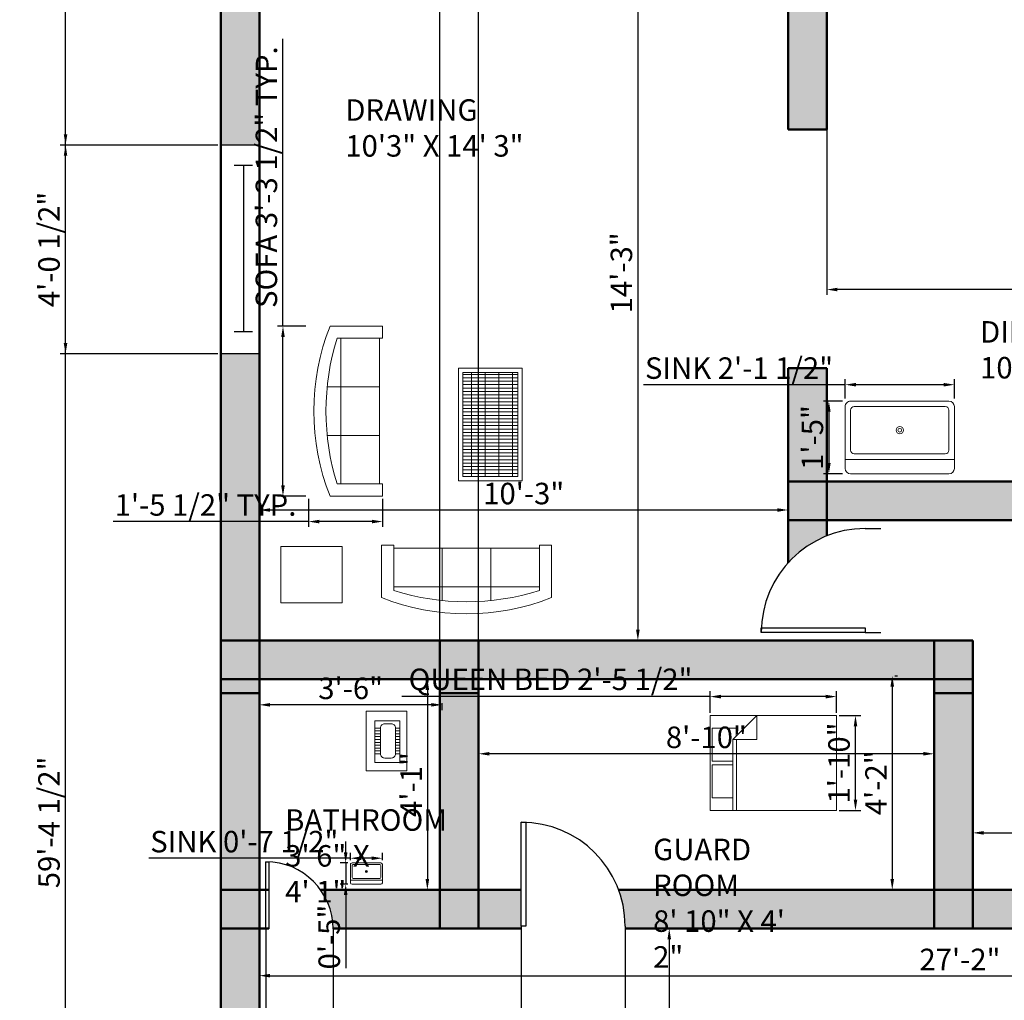
# Model space of a CAD drawing. Units: millimetres. Extents: x 2784 to 3697, y 603 to 1406.
# Tile 2 of 10: x 2784 to 3013, y 959 to 1187. Entities that reach past the tile are written whole.
import ezdxf

# ---------------------------------------------------------------- set-up
doc = ezdxf.new("R2010")
doc.units = ezdxf.units.MM
for name, color, linetype, lineweight in [('A-ANNO-DIMS', 140, 'Continuous', 18), ('A-AREA-IDEN', 150, 'Continuous', 25), ('A-DOOR', 10, 'Continuous', 25), ('A-FLOR-FIXT', 8, 'Continuous', 18), ('A-FURN', 80, 'Continuous', 18), ('A-GLAZ', 30, 'Continuous', 25), ('A-WALL', 2, 'Continuous', 50), ('A-WALL-PATT', 8, 'Continuous', 13)]:
    doc.layers.add(name, color=color, linetype=linetype, lineweight=lineweight)
doc.styles.get("Standard").update_dxf_attribs({"font": 'arial.ttf'})
doc.dimstyles.new('ISO-25', dxfattribs={"dimtxt": 5, "dimasz": 2.5, "dimexe": 1.25, "dimexo": 0.625, "dimtad": 1, "dimdec": 0, "dimlunit": 3, "dimtxsty": 'Standard', "dimcen": 2.5, "dimadec": 0, "dimazin": 0, "dimtfac": 1, "dimtdec": 0, "dimtmove": 0, "dimatfit": 3, "dimfxl": 1, "dimarcsym": 0})

# ---------------------------------------------------------------- blocks, each defined once
blk = doc.blocks.new('*U2')
for p, q in [((0, 0), (0, -6)), ((40, 0), (40, -6))]:
    blk.add_line(p, q)
blk.add_lwpolyline([(0, 0), (0, 40), (1.75, 40), (1.75, 0)], close=True)
blk.add_arc((0, 0), 40, 0, 90)
blk = doc.blocks.new('*U4')
for p, q in [((0, 4), (0, 0)), ((36, 4), (36, 0)), ((0, 2), (36, 2))]:
    blk.add_line(p, q)
blk = doc.blocks.new('Sofa - Roundback 7 ft.')
for p, q in [((-12.00002, -32.4421), (-12.00003, -6.5971)), ((11.99997, -32.4421), (11.99998, -6.5971)), ((-36.000027, -34), (-36.000027, -11.4696)), ((-35.999844, -13.3819), (35.9998, -13.3819)), ((35.99998, -34), (35.99998, -11.4696)), ((-36.000027, -32.4421), (35.99998, -32.4421))]:
    blk.add_line(p, q)
for points in [[(-36.000027, -34), (-42.000027, -34), (-42.000027, -8)], [(41.99998, -8), (41.99998, -34), (35.99998, -34)]]:
    blk.add_lwpolyline(points)
for centre, radius, start, end in [((0, -114.25), 114.25, 68.43141, 111.5686), ((-0.00001, -127.1968), 121.1968, 72.72033, 107.2797)]:
    blk.add_arc(centre, radius, start, end)
blk = doc.blocks.new('Sink-single - 30 in top')
blk.add_line((-15, -3.999996), (15, -3.999996))
for points in [[(-13.5, 0), (13.5, 0)], [(-15, -18.499996), (-15, -1.5)], [(15, -1.5), (15, -18.499996)], [(-13.5, -17.499996), (-13.5, -6.499996)], [(-12.5, -5.499996), (12.5, -5.499996)], [(13.5, -6.499996), (13.5, -17.499996)], [(12.5, -18.499996), (-12.5, -18.499996)], [(13.5, -19.999996), (-13.5, -19.999996)]]:
    blk.add_lwpolyline(points)
for radius in [1, 0.5]:
    blk.add_circle((0, -11.999996), radius)
for centre, radius, start, end in [((-13.5, -1.5), 1.5, 90, 180), ((13.5, -1.5), 1.5, 0, 90), ((-12.5, -6.499996), 1, 90, 180), ((12.5, -6.499996), 1, 0, 90), ((-13.5, -18.499996), 1.5, 180, 270), ((-12.5, -17.499996), 1, 180, 270), ((12.5, -17.499996), 1, 270, 0), ((13.5, -18.499996), 1.5, 270, 0)]:
    blk.add_arc(centre, radius, start, end)
blk = doc.blocks.new('Bed - Queen')
for p, q in [((0, -80.00003), (0, 0)), ((0, 0), (59.99999, 0)), ((59.99999, 0), (59.99999, -80.00003)), ((7.99999, -1.2), (28.79998, -1.2)), ((7.99999, -14.4), (7.99999, -1.2)), ((28.79998, -1.2), (28.79998, -14.4)), ((31.19999, -1.2), (51.99999, -1.2)), ((31.19999, -14.4), (31.19999, -1.2)), ((51.99999, -1.2), (51.99999, -16.4)), ((0, -14.4), (44.8, -14.4)), ((44.8, -16.8), (0, -16.8)), ((59.99999, -29.6), (44.8, -14.4)), ((44.8, -14.4), (44.8, -29.6)), ((51.99999, -16.4), (46.79936, -16.4)), ((44.8, -29.6), (59.99999, -29.6)), ((59.99999, -80.00003), (0, -80.00003))]:
    blk.add_line(p, q)
blk = doc.blocks.new('*D21')
at = {"layer": 'A-ANNO-DIMS', "color": 0, "lineweight": -2, "transparency": 16777216}
for p, q in [((2927.49, 1213.23), (2929.22, 1213.23)), ((2927.97, 1210.73), (2927.97, 1044.73)), ((2927.49, 1042.23), (2929.22, 1042.23))]:
    blk.add_line(p, q, dxfattribs=at)
at = {"layer": 'A-ANNO-DIMS', "color": 0, "transparency": 16777216}
for points in [[(2927.55, 1210.73), (2928.39, 1210.73), (2927.97, 1213.23)], [(2927.55, 1044.73), (2928.39, 1044.73), (2927.97, 1042.23)]]:
    blk.add_solid(points, dxfattribs=at)
at = {"layer": 'Defpoints', "color": 0, "transparency": 16777216}
for p in [(2926.87, 1213.23), (2926.87, 1042.23), (2927.97, 1042.23)]:
    blk.add_point(p, dxfattribs=at)
at = {"layer": 'A-ANNO-DIMS', "color": 0, "transparency": 16777216, "insert": (2924.79, 1127.73), "char_height": 5, "attachment_point": 5, "rotation": 90}
blk.add_mtext('14\'-3"', dxfattribs=at)
blk = doc.blocks.new('*D22')
at = {"layer": 'A-ANNO-DIMS', "color": 0, "lineweight": -2, "transparency": 16777216}
for p, q in [((2839.91, 1073.82), (2839.91, 1071.32)), ((2960.41, 1072.57), (2842.41, 1072.57)), ((2962.91, 1073.82), (2962.91, 1071.32))]:
    blk.add_line(p, q, dxfattribs=at)
at = {"layer": 'A-ANNO-DIMS', "color": 0, "transparency": 16777216}
for points in [[(2842.41, 1072.98), (2842.41, 1072.15), (2839.91, 1072.57)], [(2960.41, 1072.98), (2960.41, 1072.15), (2962.91, 1072.57)]]:
    blk.add_solid(points, dxfattribs=at)
at = {"layer": 'Defpoints', "color": 0, "transparency": 16777216}
for p in [(2839.91, 1074.44), (2962.91, 1074.44), (2839.91, 1072.57)]:
    blk.add_point(p, dxfattribs=at)
at = {"layer": 'A-ANNO-DIMS', "color": 0, "transparency": 16777216, "insert": (2901.41, 1075.75), "char_height": 5, "attachment_point": 5}
blk.add_mtext('10\'-3"', dxfattribs=at)
blk = doc.blocks.new('*D27')
at = {"layer": 'A-ANNO-DIMS', "color": 0, "lineweight": -2, "transparency": 16777216}
for p, q in [((3005.91, 1000.77), (3005.91, 996.23)), ((3165.91, 1000.77), (3165.91, 996.23)), ((3008.41, 997.48), (3163.41, 997.48))]:
    blk.add_line(p, q, dxfattribs=at)
at = {"layer": 'A-ANNO-DIMS', "color": 0, "transparency": 16777216}
for points in [[(3008.41, 997.9), (3008.41, 997.06), (3005.91, 997.48)], [(3163.41, 997.9), (3163.41, 997.06), (3165.91, 997.48)]]:
    blk.add_solid(points, dxfattribs=at)
at = {"layer": 'Defpoints', "color": 0, "transparency": 16777216}
for p in [(3005.91, 1001.39), (3165.91, 1001.39), (3165.91, 997.48)]:
    blk.add_point(p, dxfattribs=at)
at = {"layer": 'A-ANNO-DIMS', "color": 0, "transparency": 16777216, "insert": (3085.91, 1000.66), "char_height": 5, "attachment_point": 5}
blk.add_mtext('13\'-4"', dxfattribs=at)
blk = doc.blocks.new('*D30')
at = {"layer": 'A-ANNO-DIMS', "color": 0, "lineweight": -2, "transparency": 16777216}
for p, q in [((2879.44, 1033.23), (2880.24, 1033.23)), ((2878.99, 1030.73), (2878.99, 986.73)), ((2879.44, 984.23), (2880.24, 984.23))]:
    blk.add_line(p, q, dxfattribs=at)
at = {"layer": 'A-ANNO-DIMS', "color": 0, "transparency": 16777216}
for points in [[(2878.58, 1030.73), (2879.41, 1030.73), (2878.99, 1033.23)], [(2878.58, 986.73), (2879.41, 986.73), (2878.99, 984.23)]]:
    blk.add_solid(points, dxfattribs=at)
at = {"layer": 'Defpoints', "color": 0, "transparency": 16777216}
for p in [(2878.81, 1033.23), (2878.81, 984.23), (2878.99, 984.23)]:
    blk.add_point(p, dxfattribs=at)
at = {"layer": 'A-ANNO-DIMS', "color": 0, "transparency": 16777216, "insert": (2875.86, 1008.73), "char_height": 5, "attachment_point": 5, "rotation": 90}
blk.add_mtext('4\'-1"', dxfattribs=at)
blk = doc.blocks.new('*D31')
at = {"layer": 'A-ANNO-DIMS', "color": 0, "lineweight": -2, "transparency": 16777216}
for p, q in [((2839.91, 1027.65), (2839.91, 1026.01)), ((2879.88, 1027.26), (2842.41, 1027.26)), ((2882.38, 1027.65), (2882.38, 1026.01))]:
    blk.add_line(p, q, dxfattribs=at)
at = {"layer": 'A-ANNO-DIMS', "color": 0, "transparency": 16777216}
for points in [[(2842.41, 1027.68), (2842.41, 1026.84), (2839.91, 1027.26)], [(2879.88, 1027.68), (2879.88, 1026.84), (2882.38, 1027.26)]]:
    blk.add_solid(points, dxfattribs=at)
at = {"layer": 'Defpoints', "color": 0, "transparency": 16777216}
for p in [(2839.91, 1028.28), (2839.91, 1027.26), (2882.38, 1028.28)]:
    blk.add_point(p, dxfattribs=at)
at = {"layer": 'A-ANNO-DIMS', "color": 0, "transparency": 16777216, "insert": (2861.14, 1030.44), "char_height": 5, "attachment_point": 5}
blk.add_mtext('3\'-6"', dxfattribs=at)
blk = doc.blocks.new('*D32')
at = {"layer": 'A-ANNO-DIMS', "color": 0, "lineweight": -2, "transparency": 16777216}
for p, q in [((2987.78, 1034), (2988.41, 1034)), ((2987.16, 1031.5), (2987.16, 986.73)), ((2987.78, 984.23), (2988.41, 984.23))]:
    blk.add_line(p, q, dxfattribs=at)
at = {"layer": 'A-ANNO-DIMS', "color": 0, "transparency": 16777216}
for points in [[(2986.74, 1031.5), (2987.57, 1031.5), (2987.16, 1034)], [(2986.74, 986.73), (2987.57, 986.73), (2987.16, 984.23)]]:
    blk.add_solid(points, dxfattribs=at)
at = {"layer": 'Defpoints', "color": 0, "transparency": 16777216}
for p in [(2987.15, 1034), (2987.15, 984.23), (2987.16, 984.23)]:
    blk.add_point(p, dxfattribs=at)
at = {"layer": 'A-ANNO-DIMS', "color": 0, "transparency": 16777216, "insert": (2984.02, 1009.12), "char_height": 5, "attachment_point": 5, "rotation": 90}
blk.add_mtext('4\'-2"', dxfattribs=at)
blk = doc.blocks.new('*D33')
at = {"layer": 'A-ANNO-DIMS', "color": 0, "lineweight": -2, "transparency": 16777216}
for p, q in [((2890.91, 1016.5), (2890.91, 1017.12)), ((2994.41, 1015.87), (2893.41, 1015.87)), ((2996.91, 1013.48), (2996.91, 1017.12))]:
    blk.add_line(p, q, dxfattribs=at)
at = {"layer": 'A-ANNO-DIMS', "color": 0, "transparency": 16777216}
for points in [[(2893.41, 1016.29), (2893.41, 1015.46), (2890.91, 1015.87)], [(2994.41, 1016.29), (2994.41, 1015.46), (2996.91, 1015.87)]]:
    blk.add_solid(points, dxfattribs=at)
at = {"layer": 'Defpoints', "color": 0, "transparency": 16777216}
for p in [(2890.91, 1015.87), (2890.91, 1015.87), (2996.91, 1012.85)]:
    blk.add_point(p, dxfattribs=at)
at = {"layer": 'A-ANNO-DIMS', "color": 0, "transparency": 16777216, "insert": (2943.91, 1019.05), "char_height": 5, "attachment_point": 5}
blk.add_mtext('8\'-10"', dxfattribs=at)
blk = doc.blocks.new('*D34')
at = {"layer": 'A-ANNO-DIMS', "color": 0, "lineweight": -2, "transparency": 16777216}
for p, q in [((2935.34, 975.23), (2936.52, 975.23)), ((2935.27, 972.73), (2935.27, 727.73)), ((2935.34, 725.23), (2936.52, 725.23))]:
    blk.add_line(p, q, dxfattribs=at)
at = {"layer": 'A-ANNO-DIMS', "color": 0, "transparency": 16777216}
for points in [[(2934.85, 972.73), (2935.69, 972.73), (2935.27, 975.23)], [(2934.85, 727.73), (2935.69, 727.73), (2935.27, 725.23)]]:
    blk.add_solid(points, dxfattribs=at)
at = {"layer": 'Defpoints', "color": 0, "transparency": 16777216}
for p in [(2934.71, 975.23), (2934.71, 725.23), (2935.27, 725.23)]:
    blk.add_point(p, dxfattribs=at)
at = {"layer": 'A-ANNO-DIMS', "color": 0, "transparency": 16777216, "insert": (2932.09, 850.23), "char_height": 5, "attachment_point": 5, "rotation": 90}
blk.add_mtext('20\'-10"', dxfattribs=at)
blk = doc.blocks.new('*D35')
at = {"layer": 'A-ANNO-DIMS', "color": 0, "lineweight": -2, "transparency": 16777216}
for p, q in [((2839.91, 959.54), (2839.91, 965.51)), ((3165.91, 959.54), (3165.91, 965.51)), ((2842.41, 964.26), (3163.41, 964.26))]:
    blk.add_line(p, q, dxfattribs=at)
at = {"layer": 'A-ANNO-DIMS', "color": 0, "transparency": 16777216}
for points in [[(2842.41, 964.68), (2842.41, 963.84), (2839.91, 964.26)], [(3163.41, 964.68), (3163.41, 963.84), (3165.91, 964.26)]]:
    blk.add_solid(points, dxfattribs=at)
at = {"layer": 'Defpoints', "color": 0, "transparency": 16777216}
for p in [(3165.91, 964.26), (2839.91, 958.92), (3165.91, 958.92)]:
    blk.add_point(p, dxfattribs=at)
at = {"layer": 'A-ANNO-DIMS', "color": 0, "transparency": 16777216, "insert": (3002.91, 967.39), "char_height": 5, "attachment_point": 5}
blk.add_mtext('27\'-2"', dxfattribs=at)
blk = doc.blocks.new('*D36')
at = {"layer": 'A-ANNO-DIMS', "color": 0, "lineweight": -2, "transparency": 16777216}
for p, q in [((2971.91, 1166.33), (2971.91, 1122.59)), ((3096.91, 1166.33), (3096.91, 1122.59)), ((3094.41, 1123.84), (2974.41, 1123.84))]:
    blk.add_line(p, q, dxfattribs=at)
at = {"layer": 'A-ANNO-DIMS', "color": 0, "transparency": 16777216}
for points in [[(2974.41, 1124.26), (2974.41, 1123.43), (2971.91, 1123.84)], [(3094.41, 1124.26), (3094.41, 1123.43), (3096.91, 1123.84)]]:
    blk.add_solid(points, dxfattribs=at)
at = {"layer": 'Defpoints', "color": 0, "transparency": 16777216}
for p in [(2971.91, 1166.96), (3096.91, 1166.96), (2971.91, 1123.84)]:
    blk.add_point(p, dxfattribs=at)
at = {"layer": 'A-ANNO-DIMS', "color": 0, "transparency": 16777216, "insert": (3034.41, 1127.02), "char_height": 5, "attachment_point": 5}
blk.add_mtext('10\'-5"', dxfattribs=at)
blk = doc.blocks.new('*D62')
at = {"layer": 'A-ANNO-DIMS', "color": 0, "lineweight": -2, "transparency": 16777216}
for p, q in [((2944.78, 1029.17), (2873.02, 1029.17)), ((2944.78, 1025.39), (2944.78, 1030.42)), ((2971.69, 1029.17), (2947.28, 1029.17)), ((2974.19, 1025.39), (2974.19, 1030.42))]:
    blk.add_line(p, q, dxfattribs=at)
at = {"layer": 'A-ANNO-DIMS', "color": 0, "transparency": 16777216}
for points in [[(2947.28, 1029.59), (2947.28, 1028.75), (2944.78, 1029.17)], [(2971.69, 1029.59), (2971.69, 1028.75), (2974.19, 1029.17)]]:
    blk.add_solid(points, dxfattribs=at)
at = {"layer": 'Defpoints', "color": 0, "transparency": 16777216}
for p in [(2944.78, 1029.17), (2944.78, 1024.76), (2974.19, 1024.76)]:
    blk.add_point(p, dxfattribs=at)
at = {"layer": 'A-ANNO-DIMS', "color": 0, "transparency": 16777216, "insert": (2907.65, 1032.54), "char_height": 5, "attachment_point": 5}
blk.add_mtext('QUEEN BED 2\'-5 1/2"', dxfattribs=at)
blk = doc.blocks.new('*D63')
at = {"layer": 'A-ANNO-DIMS', "color": 0, "lineweight": -2, "transparency": 16777216}
for p, q in [((2974.82, 1024.76), (2979.85, 1024.76)), ((2978.6, 1005.2), (2978.6, 1022.26)), ((2974.82, 1002.7), (2979.85, 1002.7))]:
    blk.add_line(p, q, dxfattribs=at)
at = {"layer": 'A-ANNO-DIMS', "color": 0, "transparency": 16777216}
for points in [[(2978.19, 1022.26), (2979.02, 1022.26), (2978.6, 1024.76)], [(2978.19, 1005.2), (2979.02, 1005.2), (2978.6, 1002.7)]]:
    blk.add_solid(points, dxfattribs=at)
at = {"layer": 'Defpoints', "color": 0, "transparency": 16777216}
for p in [(2974.19, 1024.76), (2978.6, 1024.76), (2974.19, 1002.7)]:
    blk.add_point(p, dxfattribs=at)
at = {"layer": 'A-ANNO-DIMS', "color": 0, "transparency": 16777216, "insert": (2975.42, 1013.73), "char_height": 5, "attachment_point": 5, "rotation": 90}
blk.add_mtext('1\'-10"', dxfattribs=at)
blk = doc.blocks.new('*D64')
at = {"layer": 'A-ANNO-DIMS', "color": 0, "lineweight": -2, "transparency": 16777216}
for p, q in [((2976.21, 1098.53), (2976.21, 1102.97)), ((3001.61, 1098.53), (3001.61, 1102.97)), ((2976.21, 1101.72), (2929.3, 1101.72)), ((2999.11, 1101.72), (2978.71, 1101.72))]:
    blk.add_line(p, q, dxfattribs=at)
at = {"layer": 'A-ANNO-DIMS', "color": 0, "transparency": 16777216}
for points in [[(2978.71, 1102.13), (2978.71, 1101.3), (2976.21, 1101.72)], [(2999.11, 1102.13), (2999.11, 1101.3), (3001.61, 1101.72)]]:
    blk.add_solid(points, dxfattribs=at)
at = {"layer": 'Defpoints', "color": 0, "transparency": 16777216}
for p in [(2976.21, 1101.72), (2976.21, 1097.91), (3001.61, 1097.91)]:
    blk.add_point(p, dxfattribs=at)
at = {"layer": 'A-ANNO-DIMS', "color": 0, "transparency": 16777216, "insert": (2951.51, 1104.93), "char_height": 5, "attachment_point": 5}
blk.add_mtext('SINK 2\'-1 1/2"', dxfattribs=at)
blk = doc.blocks.new('*D65')
at = {"layer": 'A-ANNO-DIMS', "color": 0, "lineweight": -2, "transparency": 16777216}
for p, q in [((2975.59, 1097.91), (2971.15, 1097.91)), ((2972.4, 1095.41), (2972.4, 1083.47)), ((2975.59, 1080.97), (2971.15, 1080.97))]:
    blk.add_line(p, q, dxfattribs=at)
at = {"layer": 'A-ANNO-DIMS', "color": 0, "transparency": 16777216}
for points in [[(2971.99, 1095.41), (2972.82, 1095.41), (2972.4, 1097.91)], [(2971.99, 1083.47), (2972.82, 1083.47), (2972.4, 1080.97)]]:
    blk.add_solid(points, dxfattribs=at)
at = {"layer": 'Defpoints', "color": 0, "transparency": 16777216}
for p in [(2976.21, 1097.91), (2972.4, 1080.97), (2976.21, 1080.97)]:
    blk.add_point(p, dxfattribs=at)
at = {"layer": 'A-ANNO-DIMS', "color": 0, "transparency": 16777216, "insert": (2969.23, 1089.44), "char_height": 5, "attachment_point": 5, "rotation": 90}
blk.add_mtext('1\'-5"', dxfattribs=at)
blk = doc.blocks.new('*D68')
at = {"layer": 'A-ANNO-DIMS', "color": 0, "lineweight": -2, "transparency": 16777216}
for p, q in [((2861.1, 991.09), (2861.1, 992.83)), ((2868.52, 991.09), (2868.52, 992.83)), ((2861.1, 991.58), (2814.19, 991.58)), ((2866.02, 991.58), (2863.6, 991.58))]:
    blk.add_line(p, q, dxfattribs=at)
at = {"layer": 'A-ANNO-DIMS', "color": 0, "transparency": 16777216}
for points in [[(2863.6, 992), (2863.6, 991.16), (2861.1, 991.58)], [(2866.02, 992), (2866.02, 991.16), (2868.52, 991.58)]]:
    blk.add_solid(points, dxfattribs=at)
at = {"layer": 'Defpoints', "color": 0, "transparency": 16777216}
for p in [(2861.1, 991.58), (2861.1, 990.47), (2868.52, 990.47)]:
    blk.add_point(p, dxfattribs=at)
at = {"layer": 'A-ANNO-DIMS', "color": 0, "transparency": 16777216, "insert": (2836.4, 994.79), "char_height": 5, "attachment_point": 5}
blk.add_mtext('SINK 0\'-7 1/2"', dxfattribs=at)
blk = doc.blocks.new('*D69')
at = {"layer": 'A-ANNO-DIMS', "color": 0, "lineweight": -2, "transparency": 16777216}
for p, q in [((2859.99, 992.97), (2859.99, 995.47)), ((2860.48, 990.47), (2858.74, 990.47)), ((2859.99, 990.47), (2859.99, 985.52)), ((2860.48, 985.52), (2858.74, 985.52)), ((2859.99, 983.02), (2859.99, 965.98))]:
    blk.add_line(p, q, dxfattribs=at)
at = {"layer": 'A-ANNO-DIMS', "color": 0, "transparency": 16777216}
for points in [[(2859.57, 992.97), (2860.41, 992.97), (2859.99, 990.47)], [(2859.57, 983.02), (2860.41, 983.02), (2859.99, 985.52)]]:
    blk.add_solid(points, dxfattribs=at)
at = {"layer": 'Defpoints', "color": 0, "transparency": 16777216}
for p in [(2861.1, 990.47), (2859.99, 985.52), (2861.1, 985.52)]:
    blk.add_point(p, dxfattribs=at)
at = {"layer": 'A-ANNO-DIMS', "color": 0, "transparency": 16777216, "insert": (2856.81, 973.25), "char_height": 5, "attachment_point": 5, "rotation": 90}
blk.add_mtext('0\'-5"', dxfattribs=at)
blk = doc.blocks.new('*D70')
at = {"layer": 'A-ANNO-DIMS', "color": 0, "lineweight": -2, "transparency": 16777216}
for p, q in [((2845.4, 1115.33), (2845.4, 1182.14)), ((2850.7, 1115.33), (2844.15, 1115.33)), ((2845.4, 1078.31), (2845.4, 1112.83)), ((2850.7, 1075.81), (2844.15, 1075.81))]:
    blk.add_line(p, q, dxfattribs=at)
at = {"layer": 'A-ANNO-DIMS', "color": 0, "transparency": 16777216}
for points in [[(2844.98, 1112.83), (2845.82, 1112.83), (2845.4, 1115.33)], [(2844.98, 1078.31), (2845.82, 1078.31), (2845.4, 1075.81)]]:
    blk.add_solid(points, dxfattribs=at)
at = {"layer": 'Defpoints', "color": 0, "transparency": 16777216}
for p in [(2845.4, 1115.33), (2851.33, 1115.33), (2851.33, 1075.81)]:
    blk.add_point(p, dxfattribs=at)
at = {"layer": 'A-ANNO-DIMS', "color": 0, "transparency": 16777216, "insert": (2842.19, 1149.99), "char_height": 5, "attachment_point": 5, "rotation": 90}
blk.add_mtext('SOFA 3\'-3 1/2" TYP.', dxfattribs=at)
blk = doc.blocks.new('*D71')
at = {"layer": 'A-ANNO-DIMS', "color": 0, "lineweight": -2, "transparency": 16777216}
for p, q in [((2851.33, 1075.18), (2851.33, 1068.63)), ((2868.58, 1075.18), (2868.58, 1068.63)), ((2851.33, 1069.88), (2805.92, 1069.88)), ((2866.08, 1069.88), (2853.83, 1069.88))]:
    blk.add_line(p, q, dxfattribs=at)
at = {"layer": 'A-ANNO-DIMS', "color": 0, "transparency": 16777216}
for points in [[(2853.83, 1070.3), (2853.83, 1069.46), (2851.33, 1069.88)], [(2866.08, 1070.3), (2866.08, 1069.46), (2868.58, 1069.88)]]:
    blk.add_solid(points, dxfattribs=at)
at = {"layer": 'Defpoints', "color": 0, "transparency": 16777216}
for p in [(2851.33, 1075.81), (2868.58, 1075.81), (2851.33, 1069.88)]:
    blk.add_point(p, dxfattribs=at)
at = {"layer": 'A-ANNO-DIMS', "color": 0, "transparency": 16777216, "insert": (2827.38, 1073.09), "char_height": 5, "attachment_point": 5, "rotation": 0}
blk.add_mtext('1\'-5 1/2" TYP.', dxfattribs=at)
blk = doc.blocks.new('*D86')
at = {"layer": 'A-ANNO-DIMS', "color": 0, "lineweight": -2, "transparency": 16777216}
for p, q in [((2830.28, 1157.46), (2793.56, 1157.46)), ((2794.81, 1111.38), (2794.81, 1154.96)), ((2830.28, 1108.88), (2793.56, 1108.88))]:
    blk.add_line(p, q, dxfattribs=at)
at = {"layer": 'A-ANNO-DIMS', "color": 0, "transparency": 16777216}
for points in [[(2794.39, 1154.96), (2795.22, 1154.96), (2794.81, 1157.46)], [(2794.39, 1111.38), (2795.22, 1111.38), (2794.81, 1108.88)]]:
    blk.add_solid(points, dxfattribs=at)
at = {"layer": 'Defpoints', "color": 0, "transparency": 16777216}
for p in [(2794.81, 1157.46), (2830.91, 1157.46), (2830.91, 1108.88)]:
    blk.add_point(p, dxfattribs=at)
at = {"layer": 'A-ANNO-DIMS', "color": 0, "transparency": 16777216, "insert": (2791.6, 1133.17), "char_height": 5, "attachment_point": 5, "rotation": 90}
blk.add_mtext('4\'-0 1/2"', dxfattribs=at)
blk = doc.blocks.new('*D87')
at = {"layer": 'A-ANNO-DIMS', "color": 0, "lineweight": -2, "transparency": 16777216}
for p, q in [((2830.28, 1268.19), (2793.56, 1268.19)), ((2794.81, 1159.96), (2794.81, 1265.69)), ((2830.28, 1157.46), (2793.56, 1157.46))]:
    blk.add_line(p, q, dxfattribs=at)
at = {"layer": 'A-ANNO-DIMS', "color": 0, "transparency": 16777216}
for points in [[(2794.39, 1265.69), (2795.22, 1265.69), (2794.81, 1268.19)], [(2794.39, 1159.96), (2795.22, 1159.96), (2794.81, 1157.46)]]:
    blk.add_solid(points, dxfattribs=at)
at = {"layer": 'Defpoints', "color": 0, "transparency": 16777216}
for p in [(2794.81, 1268.19), (2830.91, 1268.19), (2830.91, 1157.46)]:
    blk.add_point(p, dxfattribs=at)
at = {"layer": 'A-ANNO-DIMS', "color": 0, "transparency": 16777216, "insert": (2791.6, 1212.82), "char_height": 5, "attachment_point": 5, "rotation": 90}
blk.add_mtext('9\'-2 1/2"', dxfattribs=at)
blk = doc.blocks.new('*D90')
at = {"layer": 'A-ANNO-DIMS', "color": 0, "lineweight": -2, "transparency": 16777216}
for p, q in [((2830.28, 1356.23), (2793.56, 1356.23)), ((2794.81, 646.1), (2794.81, 1353.73)), ((2830.28, 643.6), (2793.56, 643.6))]:
    blk.add_line(p, q, dxfattribs=at)
at = {"layer": 'A-ANNO-DIMS', "color": 0, "transparency": 16777216}
for points in [[(2794.39, 1353.73), (2795.22, 1353.73), (2794.81, 1356.23)], [(2794.39, 646.1), (2795.22, 646.1), (2794.81, 643.6)]]:
    blk.add_solid(points, dxfattribs=at)
at = {"layer": 'Defpoints', "color": 0, "transparency": 16777216}
for p in [(2794.81, 1356.23), (2830.91, 1356.23), (2830.91, 643.6)]:
    blk.add_point(p, dxfattribs=at)
at = {"layer": 'A-ANNO-DIMS', "color": 0, "transparency": 16777216, "insert": (2791.6, 999.91), "char_height": 5, "attachment_point": 5, "rotation": 90}
blk.add_mtext('59\'-4 1/2"', dxfattribs=at)
blk = doc.blocks.new('*D102')
at = {"layer": 'A-ANNO-DIMS', "color": 0, "lineweight": -2, "transparency": 16777216}
for p, q in [((2841.43, 974.52), (2841.43, 606.25)), ((2857.05, 974.52), (2857.05, 606.25)), ((2843.93, 607.5), (2854.55, 607.5)), ((2857.05, 607.5), (2885.27, 607.5))]:
    blk.add_line(p, q, dxfattribs=at)
at = {"layer": 'A-ANNO-DIMS', "color": 0, "transparency": 16777216}
for points in [[(2843.93, 607.91), (2843.93, 607.08), (2841.43, 607.5)], [(2854.55, 607.91), (2854.55, 607.08), (2857.05, 607.5)]]:
    blk.add_solid(points, dxfattribs=at)
at = {"layer": 'Defpoints', "color": 0, "transparency": 16777216}
for p in [(2841.43, 975.14), (2857.05, 975.14), (2857.05, 607.5)]:
    blk.add_point(p, dxfattribs=at)
at = {"layer": 'A-ANNO-DIMS', "color": 0, "transparency": 16777216, "insert": (2872.41, 610.71), "char_height": 5, "attachment_point": 5}
blk.add_mtext('1\'-3 1/2"', dxfattribs=at)
blk = doc.blocks.new('*D103')
at = {"layer": 'A-ANNO-DIMS', "color": 0, "lineweight": -2, "transparency": 16777216}
for p, q in [((2900.85, 974.61), (2900.85, 606.25)), ((2925.01, 974.61), (2925.01, 606.25)), ((2903.35, 607.5), (2922.51, 607.5))]:
    blk.add_line(p, q, dxfattribs=at)
at = {"layer": 'A-ANNO-DIMS', "color": 0, "transparency": 16777216}
for points in [[(2903.35, 607.91), (2903.35, 607.08), (2900.85, 607.5)], [(2922.51, 607.91), (2922.51, 607.08), (2925.01, 607.5)]]:
    blk.add_solid(points, dxfattribs=at)
at = {"layer": 'Defpoints', "color": 0, "transparency": 16777216}
for p in [(2900.85, 975.23), (2925.01, 975.23), (2925.01, 607.5)]:
    blk.add_point(p, dxfattribs=at)
at = {"layer": 'A-ANNO-DIMS', "color": 0, "transparency": 16777216, "insert": (2912.93, 610.67), "char_height": 5, "attachment_point": 5}
blk.add_mtext('2\'-0"', dxfattribs=at)
blk = doc.blocks.new('*D104')
at = {"layer": 'A-ANNO-DIMS', "color": 0, "lineweight": -2, "transparency": 16777216}
for p, q in [((2881.91, 1030.6), (2881.91, 1393.58)), ((2890.91, 1030.6), (2890.91, 1393.58)), ((2884.41, 1392.33), (2888.41, 1392.33)), ((2890.91, 1392.33), (2907.95, 1392.33))]:
    blk.add_line(p, q, dxfattribs=at)
at = {"layer": 'A-ANNO-DIMS', "color": 0, "transparency": 16777216}
for points in [[(2884.41, 1392.75), (2884.41, 1391.91), (2881.91, 1392.33)], [(2888.41, 1392.75), (2888.41, 1391.91), (2890.91, 1392.33)]]:
    blk.add_solid(points, dxfattribs=at)
at = {"layer": 'Defpoints', "color": 0, "transparency": 16777216}
for p in [(2890.91, 1392.33), (2881.91, 1029.97), (2890.91, 1029.97)]:
    blk.add_point(p, dxfattribs=at)
at = {"layer": 'A-ANNO-DIMS', "color": 0, "transparency": 16777216, "insert": (2900.68, 1395.51), "char_height": 5, "attachment_point": 5}
blk.add_mtext('0\'-9"', dxfattribs=at)

msp = doc.modelspace()

# ---------------------------------------------------------------- hatches: boundary and pattern name
at = {"layer": 'A-FURN'}
h = msp.add_hatch(dxfattribs=at)
h.set_pattern_fill('GRATE', color=256)
h.paths.add_polyline_path([(2900.03, 1104.57), (2887.22, 1104.57), (2887.22, 1080.38), (2900.03, 1080.38)])
at = {"layer": 'A-WALL-PATT'}
h = msp.add_hatch(color=256, dxfattribs=at)
h.dxf.hatch_style = 1
h.paths.add_polyline_path([(2869.53, 1356.23), (2839.91, 1356.23), (2839.91, 1347.23), (2869.53, 1347.23)])
h.paths.add_polyline_path([(2839.91, 1356.23), (2830.91, 1356.23), (2830.91, 1347.23), (2839.91, 1347.23)])
h.paths.add_polyline_path([(2839.91, 1347.23), (2830.91, 1347.23), (2830.91, 1314.23), (2839.91, 1314.23)])
h.paths.add_polyline_path([(2839.91, 1268.19), (2830.91, 1268.19), (2830.91, 1222.23), (2839.91, 1222.23)])
h.paths.add_polyline_path([(2839.91, 1222.23), (2830.91, 1222.23), (2830.91, 1213.23), (2839.91, 1213.23)])
h.paths.add_polyline_path([(2962.91, 1222.23), (2839.91, 1222.23), (2839.91, 1213.23), (2962.91, 1213.23)])
h.paths.add_polyline_path([(2971.91, 1222.23), (2962.91, 1222.23), (2962.91, 1213.23), (2971.91, 1213.23)])
h.paths.add_polyline_path([(2971.91, 1263.23), (2962.91, 1263.23), (2962.91, 1254.23), (2971.91, 1254.23)])
h.paths.add_polyline_path([(2971.91, 1347.23), (2962.91, 1347.23), (2962.91, 1263.23), (2971.91, 1263.23)])
h.paths.add_polyline_path([(2971.91, 1356.23), (2962.91, 1356.23), (2962.91, 1347.23), (2971.91, 1347.23)])
h.paths.add_polyline_path([(2962.91, 1356.23), (2913.7, 1356.23), (2913.7, 1347.23), (2962.91, 1347.23)])
h.paths.add_polyline_path([(2982.62, 1356.23), (2971.91, 1356.23), (2971.91, 1347.23), (2982.62, 1347.23)])
h.paths.add_polyline_path([(3019.91, 1356.23), (3004.44, 1356.23), (3004.44, 1347.23), (3019.91, 1347.23)])
h.paths.add_polyline_path([(3028.91, 1356.23), (3019.91, 1356.23), (3019.91, 1347.23), (3028.91, 1347.23)])
h.paths.add_polyline_path([(3028.91, 1347.23), (3019.91, 1347.23), (3019.91, 1287.35, -0.06506), (3026.12, 1288.16), (3028.91, 1288.16)])
h.paths.add_polyline_path([(3019.91, 1263.23), (2971.91, 1263.23), (2971.91, 1254.23), (3019.91, 1254.23)])
h.paths.add_polyline_path([(3028.91, 1263.23), (3019.91, 1263.23), (3019.91, 1254.23), (3028.91, 1254.23)])
h.paths.add_polyline_path([(3028.91, 1254.23), (3019.91, 1254.23), (3019.91, 1222.23), (3028.91, 1222.23)])
h.paths.add_polyline_path([(3028.91, 1222.23), (3019.91, 1222.23), (3019.91, 1213.23), (3028.91, 1213.23)])
h.paths.add_polyline_path([(3165.91, 1222.23), (3060.65, 1222.23, -0.056956), (3061.45, 1215.23), (3061.45, 1213.23), (3165.91, 1213.23)])
h.paths.add_polyline_path([(3080.34, 1356.23), (3028.91, 1356.23), (3028.91, 1347.23), (3080.34, 1347.23)])
h.paths.add_polyline_path([(3174.91, 1347.23), (3165.91, 1347.23), (3165.91, 1311.28), (3174.91, 1311.28)])
h.paths.add_polyline_path([(3174.91, 1356.23), (3165.91, 1356.23), (3165.91, 1347.23), (3174.91, 1347.23)])
h.paths.add_polyline_path([(3165.91, 1356.23), (3123.1, 1356.23), (3123.1, 1347.23), (3165.91, 1347.23)])
h.paths.add_polyline_path([(3174.91, 1266.65), (3165.91, 1266.65), (3165.91, 1222.23), (3174.91, 1222.23)])
h.paths.add_polyline_path([(3174.91, 1222.23), (3165.91, 1222.23), (3165.91, 1213.23), (3174.91, 1213.23)])
h.paths.add_polyline_path([(3174.91, 1213.23), (3165.91, 1213.23), (3165.91, 1194.83), (3174.91, 1194.83)])
h.paths.add_polyline_path([(3105.91, 1182.92, -0.096276), (3096.91, 1180.92), (3096.91, 1148.23), (3105.91, 1148.23)])
h.paths.add_polyline_path([(3105.91, 1213.23), (3096.91, 1213.23), (3096.91, 1205.07), (3105.91, 1205.07)])
h.paths.add_polyline_path([(2971.91, 1213.23), (2962.91, 1213.23), (2962.91, 1161.09), (2971.91, 1161.09)])
h.paths.add_polyline_path([(2839.91, 1213.23), (2830.91, 1213.23), (2830.91, 1157.46), (2839.91, 1157.46)])
h.paths.add_polyline_path([(2839.91, 1108.88), (2830.91, 1108.88), (2830.91, 1042.23), (2839.91, 1042.23)])
h.paths.add_polyline_path([(2839.91, 1042.23), (2830.91, 1042.23), (2830.91, 1033.23), (2839.91, 1033.23)])
h.paths.add_polyline_path([(2881.91, 1042.23), (2839.91, 1042.23), (2839.91, 1033.23), (2881.91, 1033.23)])
h.paths.add_polyline_path([(2996.91, 1042.23), (2890.91, 1042.23), (2890.91, 1033.23), (2996.91, 1033.23)])
h.paths.add_polyline_path([(2890.91, 1042.23), (2881.91, 1042.23), (2881.91, 1033.23), (2890.91, 1033.23)])
h.paths.add_polyline_path([(2890.91, 1033.23), (2881.91, 1033.23), (2881.91, 984.23), (2890.91, 984.23)])
h.paths.add_polyline_path([(2839.91, 1033.23), (2830.91, 1033.23), (2830.91, 984.23), (2839.91, 984.23)])
h.paths.add_polyline_path([(2839.91, 984.23), (2830.91, 984.23), (2830.91, 975.23), (2839.91, 975.23)])
h.paths.add_polyline_path([(2881.91, 984.23), (2854.14, 984.23, -0.154991), (2857.05, 975.23), (2881.91, 975.23)])
h.paths.add_polyline_path([(2890.91, 984.23), (2881.91, 984.23), (2881.91, 975.23), (2890.91, 975.23)])
h.paths.add_polyline_path([(2900.85, 984.23), (2890.91, 984.23), (2890.91, 975.23), (2900.85, 975.23), (2900.85, 975.78)])
h.paths.add_polyline_path([(2996.91, 984.23), (2923.49, 984.23, -0.089525), (2925.01, 975.78), (2925.01, 975.23), (2996.91, 975.23)])
h.paths.add_polyline_path([(3165.91, 984.23), (3005.91, 984.23), (3005.91, 975.23), (3165.91, 975.23)])
h.paths.add_polyline_path([(3005.91, 1033.23), (2996.91, 1033.23), (2996.91, 984.23), (3005.91, 984.23)])
h.paths.add_polyline_path([(3005.91, 984.23), (2996.91, 984.23), (2996.91, 975.23), (3005.91, 975.23)])
h.paths.add_polyline_path([(3005.91, 1042.23), (2996.91, 1042.23), (2996.91, 1033.23), (3005.91, 1033.23)])
h.paths.add_polyline_path([(3096.91, 1079.23), (2971.91, 1079.23), (2971.91, 1070.23), (3096.91, 1070.23)])
h.paths.add_polyline_path([(2971.91, 1079.23), (2962.91, 1079.23), (2962.91, 1070.23), (2971.91, 1070.23)])
h.paths.add_polyline_path([(2971.91, 1070.23), (2962.91, 1070.23), (2962.91, 1060.28, -0.115005), (2971.91, 1066.55)])
h.paths.add_polyline_path([(2971.91, 1105.54), (2962.91, 1105.54), (2962.91, 1079.23), (2971.91, 1079.23)])
h.paths.add_polyline_path([(3165.91, 1079.23), (3105.91, 1079.23), (3105.91, 1070.23), (3165.91, 1070.23)])
h.paths.add_polyline_path([(3105.91, 1079.23), (3096.91, 1079.23), (3096.91, 1070.23), (3105.91, 1070.23)])
h.paths.add_polyline_path([(3105.91, 1148.23), (3096.91, 1148.23), (3096.91, 1139.23), (3105.91, 1139.23)])
h.paths.add_polyline_path([(3105.91, 1139.23), (3096.91, 1139.23), (3096.91, 1104.7), (3098.08, 1104.75, -0.08216), (3105.91, 1103.81)])
h.paths.add_polyline_path([(3165.91, 1148.23), (3105.91, 1148.23), (3105.91, 1139.23), (3165.91, 1139.23)])
h.paths.add_polyline_path([(3174.91, 1148.23), (3165.91, 1148.23), (3165.91, 1139.23), (3174.91, 1139.23)])
h.paths.add_polyline_path([(3174.91, 1139.23), (3165.91, 1139.23), (3165.91, 1123.86), (3174.91, 1123.86)])
h.paths.add_polyline_path([(3174.91, 1097.37), (3165.91, 1097.37), (3165.91, 1079.23), (3174.91, 1079.23)])
h.paths.add_polyline_path([(3174.91, 1079.23), (3165.91, 1079.23), (3165.91, 1070.23), (3174.91, 1070.23)])
h.paths.add_polyline_path([(3174.91, 1070.23), (3165.91, 1070.23), (3165.91, 1048.77), (3174.91, 1048.77)])
h.paths.add_polyline_path([(3174.91, 1002.74), (3165.91, 1002.74), (3165.91, 984.23), (3174.91, 984.23)])
h.paths.add_polyline_path([(3174.91, 984.23), (3165.91, 984.23), (3165.91, 975.23), (3174.91, 975.23)])
h.paths.add_polyline_path([(3174.91, 975.23), (3165.91, 975.23), (3165.91, 725.23), (3174.91, 725.23)])
h.paths.add_polyline_path([(2839.91, 975.23), (2830.91, 975.23), (2830.91, 725.23), (2839.91, 725.23)])
h.paths.add_polyline_path([(3165.91, 725.23), (2839.91, 725.23), (2839.91, 716.23), (3165.91, 716.23)])
h.paths.add_polyline_path([(3174.91, 725.23), (3165.91, 725.23), (3165.91, 716.23), (3174.91, 716.23)])
h.paths.add_polyline_path([(2839.91, 725.23), (2830.91, 725.23), (2830.91, 716.23), (2839.91, 716.23)])

# ---------------------------------------------------------------- linework, layer by layer
at = {"layer": 'A-FURN'}
for p, q in [((2868.08, 1021.86), (2866.79, 1021.86)), ((2868.08, 1021.86), (2867.37, 1021.86)), ((2871.58, 1021.86), (2872.55, 1021.86)), ((2868.08, 1021.19), (2866.79, 1021.19)), ((2868.08, 1020.53), (2866.79, 1020.53)), ((2868.08, 1019.86), (2866.79, 1019.86)), ((2871.58, 1021.19), (2872.55, 1021.19)), ((2871.58, 1020.53), (2872.55, 1020.53)), ((2871.58, 1019.86), (2872.55, 1019.86)), ((2868.08, 1019.2), (2866.79, 1019.2)), ((2868.08, 1018.53), (2866.79, 1018.53)), ((2868.08, 1017.87), (2866.79, 1017.87)), ((2868.08, 1017.2), (2866.79, 1017.2)), ((2871.58, 1019.2), (2872.55, 1019.2)), ((2871.58, 1018.53), (2872.55, 1018.53)), ((2871.58, 1017.87), (2872.55, 1017.87)), ((2871.58, 1017.2), (2872.55, 1017.2)), ((2868.08, 1016.54), (2866.79, 1016.54)), ((2868.08, 1015.87), (2866.79, 1015.87)), ((2871.58, 1016.54), (2872.55, 1016.54)), ((2871.58, 1015.87), (2872.55, 1015.87)), ((2871.58, 1015.87), (2872.55, 1015.87))]:
    msp.add_line(p, q, dxfattribs=at)
for points in [[(2886.22, 1105.57), (2886.22, 1079.38), (2901.03, 1079.38), (2901.03, 1105.57)], [(2887.22, 1104.57), (2887.22, 1080.38), (2900.03, 1080.38), (2900.03, 1104.57)], [(2844.9, 1064.05), (2859.19, 1064.05), (2859.19, 1050.97), (2844.9, 1050.97)], [(2864.72, 1025.82), (2874.24, 1025.82), (2874.24, 1011.93), (2864.72, 1011.93)], [(2866.79, 1023.55), (2872.55, 1023.55), (2872.55, 1013.84), (2866.79, 1013.84)]]:
    msp.add_lwpolyline(points, close=True, dxfattribs=at)
msp.add_lwpolyline([(2869.08, 1022.86), (2870.58, 1022.86, -0.414214), (2871.58, 1021.86), (2871.58, 1015.87, -0.414214), (2870.58, 1014.87), (2869.08, 1014.87, -0.414214), (2868.08, 1015.87), (2868.08, 1021.86, -0.414214)], format="xyb", close=True, dxfattribs=at)
at = {"layer": 'A-GLAZ'}
for p, q in [((2839.91, 1157.46), (2830.91, 1157.46)), ((2839.91, 1108.88), (2830.91, 1108.88))]:
    msp.add_line(p, q, dxfattribs=at)
at = {"layer": 'A-WALL'}
for p, q in [((2830.91, 1356.23), (2830.91, 716.23)), ((2839.91, 1356.23), (2839.91, 643.6)), ((2962.91, 1222.82), (2962.91, 1161.09)), ((2971.91, 1222.82), (2971.91, 1161.09)), ((2962.91, 1161.09), (2971.91, 1161.09)), ((2971.91, 1105.54), (2962.91, 1105.54)), ((2962.91, 1105.54), (2962.91, 1060.28)), ((2971.91, 1105.54), (2971.91, 1066.55)), ((2962.91, 1079.23), (3174.91, 1079.23)), ((2962.91, 1070.23), (3174.91, 1070.23)), ((2830.91, 1042.23), (3005.91, 1042.23)), ((2881.91, 1042.23), (2881.91, 975.23)), ((2890.91, 1042.23), (2890.91, 975.23)), ((2996.91, 1042.23), (2996.91, 975.23)), ((3005.91, 1042.23), (3005.91, 975.23)), ((2830.91, 1033.23), (3005.91, 1033.23)), ((2839.91, 1029.97), (2830.91, 1029.97)), ((2890.91, 1029.97), (2881.91, 1029.97)), ((3005.91, 1029.97), (2996.91, 1029.97)), ((2830.91, 984.23), (2842.11, 984.23)), ((2854.14, 984.23), (2900.85, 984.23)), ((2923.49, 984.23), (3174.91, 984.23)), ((2830.91, 975.23), (2842.11, 975.23)), ((2857.05, 975.23), (2900.85, 975.23)), ((2925.01, 975.23), (3174.91, 975.23))]:
    msp.add_line(p, q, dxfattribs=at)

# ---------------------------------------------------------------- block references
at = {"layer": 'A-DOOR', "xscale": 0.6041131756153701, "yscale": 0.6041131756153701, "zscale": 0.6041131756153701, "rotation": 90}
msp.add_blockref('*U2', (2980.86, 1044.11), dxfattribs=at)
at = {"layer": 'A-DOOR'}
for p, xscale, yscale, zscale in [((2900.85, 975.78), 0.6041131756153701, 0.6041131756153701, 0.6041131756153701), ((2841.43, 975.14), 0.3906322045000195, 0.3906322045000195, 0.3906322045000195)]:
    msp.add_blockref('*U2', p, dxfattribs=dict(at, xscale=xscale, yscale=yscale, zscale=zscale))
at = {"layer": 'A-FLOR-FIXT', "rotation": 180}
for p, xscale, yscale, zscale in [((2988.91, 1080.97), 0.8466666666666576, 0.8466666666666576, 0.8466666666666576), ((2864.81, 985.52), 0.2473695176006166, 0.2473695176006166, 0.2473695176006166)]:
    msp.add_blockref('Sink-single - 30 in top', p, dxfattribs=dict(at, xscale=xscale, yscale=yscale, zscale=zscale))
at = {"layer": 'A-FURN'}
for name, p, xscale, yscale, zscale, rotation in [('Sofa - Roundback 7 ft.', (2852.58, 1095.57), 0.4705007744461669, 0.4705007744461669, 0.4705007744461669, 90.0000221689986), ('Sofa - Roundback 7 ft.', (2888.11, 1048.42), 0.4705007744461669, 0.4705007744461669, 0.4705007744461669, 180.0000221689986), ('Bed - Queen', (2944.78, 1002.7), 0.3675961586187321, 0.3675961586187321, 0.3675961586187321, 90)]:
    msp.add_blockref(name, p, dxfattribs=dict(at, xscale=xscale, yscale=yscale, zscale=zscale, rotation=rotation))
at = {"layer": 'A-GLAZ', "xscale": 1.074021802203067, "yscale": 1.074021802203067, "zscale": 1.074021802203067, "rotation": 270}
msp.add_blockref('*U4', (2834.03, 1152.7), dxfattribs=at)

# ---------------------------------------------------------------- texts
at = {"layer": 'A-AREA-IDEN', "char_height": 5, "attachment_point": 1}
for s, width, insert in [('DRAWING \\P10\'3" X 14\' 3"', 54.3124, (2859.9, 1168.1)), ('DINNING \\P10\'5" X 11\' 2"', 45.9891, (3007.59, 1116.5)), ('BATHROOM \\P3\' 6" X 4\' 1"', 24.1962, (2845.91, 1002.96)), ('GUARD ROOM \\P8\' 10" X 4\' 2"', 34.2617, (2931.52, 996.12))]:
    msp.add_mtext_dynamic_manual_height_columns(s, width=width, gutter_width=12.5, heights=[0], dxfattribs=dict(at, insert=insert))

# ---------------------------------------------------------------- dimensions: what is measured, and where the dimension line sits
at = {"layer": 'A-ANNO-DIMS'}
for base, p1, p2, override, picture, middle in [((2890.91, 1392.33), (2881.91, 1029.97), (2890.91, 1029.97), {"dimdec": 1, "dimlfac": 1, "dimrnd": 0, "dimzin": 1, "dimdsep": 46, "dimlunit": 4, "dimfrac": 2}, '*D104', (2900.68, 1395.51)), ((2971.91, 1123.84), (3096.91, 1166.96), (2971.91, 1166.96), {"dimclrd": 0, "dimclre": 0, "dimclrt": 0}, '*D36', (3034.41, 1127.02)), ((2839.91, 1072.57), (2962.91, 1074.44), (2839.91, 1074.44), {"dimclrd": 0, "dimclre": 0, "dimclrt": 0}, '*D22', (2901.41, 1075.75)), ((2839.91, 1027.26), (2882.38, 1028.28), (2839.91, 1028.28), {"dimclrd": 0, "dimclre": 0, "dimclrt": 0}, '*D31', (2861.14, 1030.44)), ((2890.91, 1015.87), (2996.91, 1012.85), (2890.91, 1015.87), {"dimclrd": 0, "dimclre": 0, "dimclrt": 0}, '*D33', (2943.91, 1019.05)), ((3165.91, 997.48), (3005.91, 1001.39), (3165.91, 1001.39), {"dimclrd": 0, "dimclre": 0, "dimclrt": 0}, '*D27', (3085.91, 1000.66)), ((2857.05, 607.5), (2841.43, 975.14), (2857.05, 975.14), {"dimdec": 1, "dimlfac": 1, "dimrnd": 0, "dimzin": 1, "dimdsep": 46, "dimlunit": 4, "dimfrac": 2}, '*D102', (2872.41, 610.71)), ((2925.01, 607.5), (2900.85, 975.23), (2925.01, 975.23), {"dimdec": 1, "dimlfac": 1, "dimrnd": 0, "dimzin": 1, "dimdsep": 46, "dimlunit": 4, "dimfrac": 2}, '*D103', (2912.93, 610.67)), ((3165.91, 964.26), (2839.91, 958.92), (3165.91, 958.92), {"dimclrd": 0, "dimclre": 0, "dimclrt": 0}, '*D35', (3002.91, 967.39))]:
    dim = msp.add_linear_dim(base=base, p1=p1, p2=p2, dimstyle='ISO-25', override=override, dxfattribs=at)
    dim.commit()
    dim.dimension.update_dxf_attribs({"geometry": picture, "text_midpoint": middle})
for base, p1, p2, angle, override, picture, middle in [((2794.81, 1356.23), (2830.91, 643.6), (2830.91, 1356.23), 90, {"dimdec": 1, "dimlfac": 1, "dimrnd": 0, "dimzin": 1, "dimdsep": 46, "dimlunit": 4, "dimfrac": 2}, '*D90', (2791.6, 999.91)), ((2794.81, 1268.19), (2830.91, 1157.46), (2830.91, 1268.19), 90, {"dimdec": 1, "dimlfac": 1, "dimrnd": 0, "dimzin": 1, "dimdsep": 46, "dimlunit": 4, "dimfrac": 2}, '*D87', (2791.6, 1212.82)), ((2927.97, 1042.23), (2926.87, 1213.23), (2926.87, 1042.23), 90, {"dimclrd": 0, "dimclre": 0, "dimclrt": 0}, '*D21', (2924.79, 1127.73)), ((2794.81, 1157.46), (2830.91, 1108.88), (2830.91, 1157.46), 90, {"dimdec": 1, "dimlfac": 1, "dimrnd": 0, "dimzin": 1, "dimdsep": 46, "dimlunit": 4, "dimfrac": 2}, '*D86', (2791.6, 1133.17)), ((2972.4, 1080.97), (2976.21, 1097.91), (2976.21, 1080.97), 270, {"dimdec": 1, "dimrnd": 0, "dimzin": 1, "dimlunit": 4, "dimfrac": 2}, '*D65', (2969.23, 1089.44)), ((2878.99, 984.23), (2878.81, 1033.23), (2878.81, 984.23), 90, {"dimclrd": 0, "dimclre": 0, "dimclrt": 0}, '*D30', (2875.86, 1008.73)), ((2987.16, 984.23), (2987.15, 1034), (2987.15, 984.23), 90, {"dimclrd": 0, "dimclre": 0, "dimclrt": 0}, '*D32', (2984.02, 1009.12)), ((2978.6, 1024.76), (2974.19, 1002.7), (2974.19, 1024.76), 90, {"dimdec": 1, "dimrnd": 0, "dimzin": 1, "dimlunit": 4, "dimfrac": 2}, '*D63', (2975.42, 1013.73)), ((2859.9906, 985.5201), (2861.1038, 990.4675), (2861.1038, 985.5201), 270, {"dimdec": 1, "dimrnd": 0, "dimzin": 1, "dimlunit": 4, "dimfrac": 2}, '*D69', (2856.8127, 973.2495)), ((2935.27, 725.23), (2934.71, 975.23), (2934.71, 725.23), 90, {"dimclrd": 0, "dimclre": 0, "dimclrt": 0}, '*D34', (2932.09, 850.23))]:
    dim = msp.add_linear_dim(base=base, p1=p1, p2=p2, angle=angle, dimstyle='ISO-25', override=override, dxfattribs=at)
    dim.commit()
    dim.dimension.update_dxf_attribs({"geometry": picture, "text_midpoint": middle})
for base, p1, p2, angle, text, picture, middle in [((2845.4, 1115.33), (2851.33, 1075.81), (2851.33, 1115.33), 90, 'SOFA <> TYP.', '*D70', (2842.19, 1149.99)), ((2976.21, 1101.72), (3001.61, 1097.91), (2976.21, 1097.91), 180, 'SINK <>', '*D64', (2951.51, 1104.93)), ((2851.3291, 1069.88), (2868.5808, 1075.8083), (2851.3291, 1075.8083), 180, '<> TYP.', '*D71', (2827.3753, 1073.0902)), ((2944.78, 1029.17), (2974.19, 1024.76), (2944.78, 1024.76), 180, 'QUEEN BED <>', '*D62', (2907.65, 1032.54)), ((2861.1, 991.58), (2868.52, 990.47), (2861.1, 990.47), 180, 'SINK <>', '*D68', (2836.4, 994.79))]:
    dim = msp.add_linear_dim(base=base, p1=p1, p2=p2, angle=angle, text=text, dimstyle='ISO-25', override={"dimdec": 1, "dimrnd": 0, "dimzin": 1, "dimlunit": 4, "dimfrac": 2}, dxfattribs=at)
    dim.commit()
    dim.dimension.update_dxf_attribs({"geometry": picture, "text_midpoint": middle})

doc.saveas('drawing.dxf')
